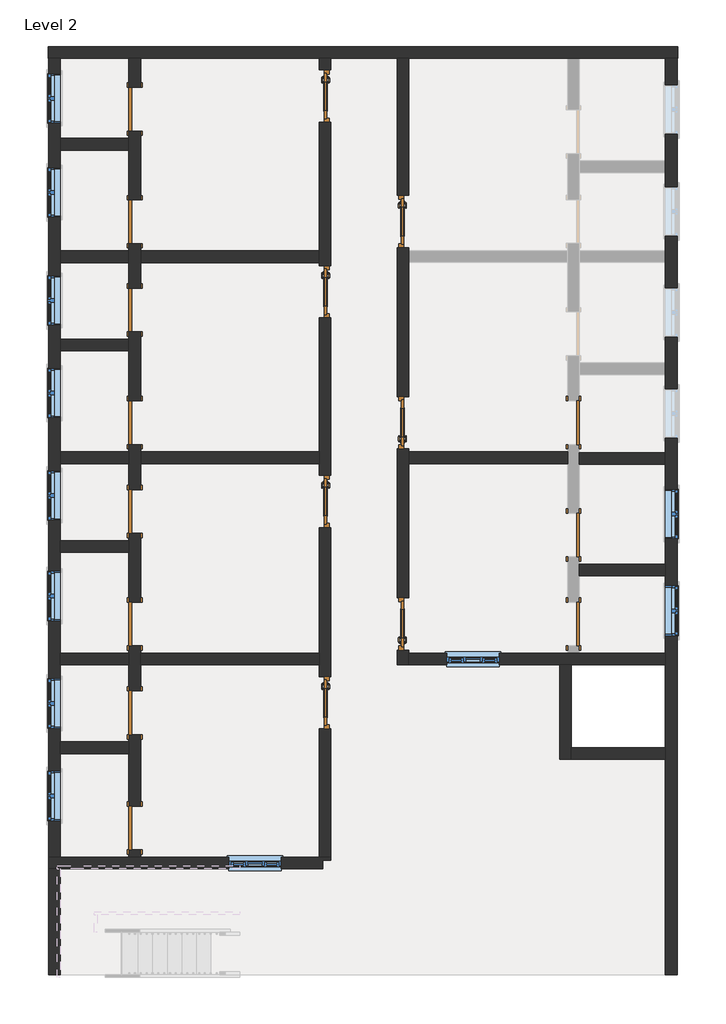
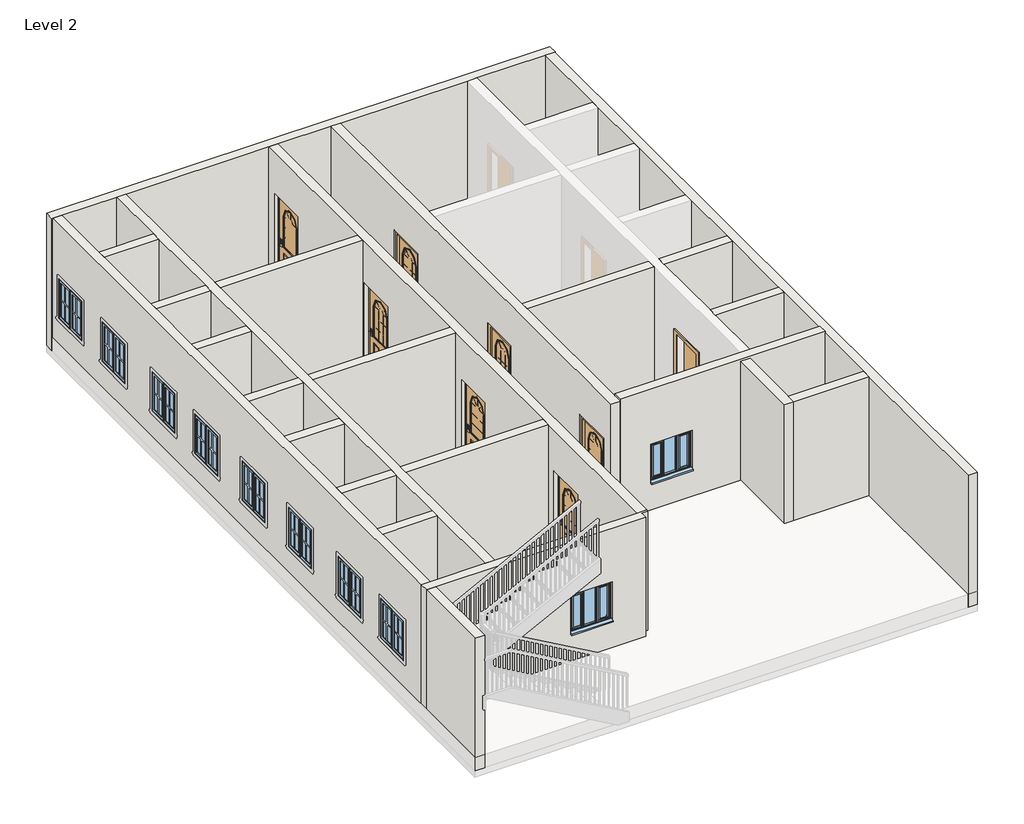
# One storey, part 1 of 4: 24 walls, 18 doors, 12 windows.
"""IFC4 building model written with IfcOpenShell, lengths in millimetres."""

from ifc_helpers import new_model, si_unit, frame, origin, place, context, project, spatial, polyline, outline, extrude, faceted_brep, transform, mapped, element, save
from components import doors_extsgl_w_glazing_bars_arched_910x2110mm_1ab485ba, doors_extsgl_w_glazing_bars_arched_910x2110mm_97dcda8a, door_fadea3f2, door_53b1b562, window_c29befe5, windows_tpl_plain_910x910mm_84e79c20

model = new_model("IFC4")

# Units and contexts
model_context = context("Model", 3, world=origin())
ifc_project = project(units=[si_unit("LENGTHUNIT", "METRE", prefix="MILLI")], contexts=[model_context])

# Site, building, storey
site = spatial("IfcSite", under=ifc_project)
building = spatial("IfcBuilding", under=site)
storey = spatial("IfcBuildingStorey", under=building, Name="Level 2", Elevation=3048.0)

# Doors
placement = place(None, origin())
doors_extsgl_w_glazing_bars_arched_910x2110mm_shape = doors_extsgl_w_glazing_bars_arched_910x2110mm_1ab485ba(model_context)
element("IfcDoor", 1, ObjectType="Doors_ExtSgl_w-Glazing_Bars_Arched : 910x2110mm", at=placement, inside=storey, context=model_context, shape_type="MappedRepresentation", body=[
    mapped(doors_extsgl_w_glazing_bars_arched_910x2110mm_shape, transform((-1635.1108866, 7135.2399728, 3048.0), x_axis=(0.0, -1.0, 0.0), y_axis=(1.0, 0.0, 0.0), z_axis=(0.0, 0.0, 1.0))),
])
element("IfcDoor", 2, ObjectType="Doors_ExtSgl_w-Glazing_Bars_Arched : 910x2110mm", at=placement, inside=storey, context=model_context, shape_type="MappedRepresentation", body=[
    mapped(doors_extsgl_w_glazing_bars_arched_910x2110mm_shape, transform((-1635.1108866, 3727.1935874, 3048.0), x_axis=(0.0, -1.0, 0.0), y_axis=(1.0, 0.0, 0.0), z_axis=(0.0, 0.0, 1.0))),
])
element("IfcDoor", 3, ObjectType="Doors_ExtSgl_w-Glazing_Bars_Arched : 910x2110mm", at=placement, inside=storey, context=model_context, shape_type="MappedRepresentation", body=[
    mapped(doors_extsgl_w_glazing_bars_arched_910x2110mm_shape, transform((-1635.1108866, 74.0399728, 3048.0), x_axis=(0.0, -1.0, 0.0), y_axis=(1.0, 0.0, 0.0), z_axis=(0.0, 0.0, 1.0))),
])
element("IfcDoor", 4, ObjectType="Doors_ExtSgl_w-Glazing_Bars_Arched : 910x2110mm", at=placement, inside=storey, context=model_context, shape_type="MappedRepresentation", body=[
    mapped(doors_extsgl_w_glazing_bars_arched_910x2110mm_shape, transform((-1635.1108866, -3431.1600272, 3048.0), x_axis=(0.0, -1.0, 0.0), y_axis=(1.0, 0.0, 0.0), z_axis=(0.0, 0.0, 1.0))),
])
element("IfcDoor", 5, ObjectType="Doors_ExtSgl_w-Glazing_Bars_Arched : 910x2110mm", at=placement, inside=storey, context=model_context, shape_type="MappedRepresentation", body=[
    mapped(doors_extsgl_w_glazing_bars_arched_910x2110mm_shape, transform((-276.2108866, -2059.5600272, 3048.0), x_axis=(0.0, 1.0, 0.0), y_axis=(-1.0, 0.0, 0.0), z_axis=(0.0, 0.0, 1.0))),
])
element("IfcDoor", 6, ObjectType="Doors_ExtSgl_w-Glazing_Bars_Arched : 910x2110mm", at=placement, inside=storey, context=model_context, shape_type="MappedRepresentation", body=[
    mapped(doors_extsgl_w_glazing_bars_arched_910x2110mm_shape, transform((-276.2108866, 1445.6399728, 3048.0), x_axis=(0.0, 1.0, 0.0), y_axis=(-1.0, 0.0, 0.0), z_axis=(0.0, 0.0, 1.0))),
])
doors_extsgl_w_glazing_bars_arched_910x2110mm_2_shape = doors_extsgl_w_glazing_bars_arched_910x2110mm_97dcda8a(model_context)
element("IfcDoor", 7, ObjectType="Doors_ExtSgl_w-Glazing_Bars_Arched : 910x2110mm", at=placement, inside=storey, context=model_context, shape_type="MappedRepresentation", body=[
    mapped(doors_extsgl_w_glazing_bars_arched_910x2110mm_2_shape, transform((-276.2108866, 4950.8399728, 3048.0), x_axis=(0.0, -1.0, 0.0), y_axis=(1.0, 0.0, 0.0), z_axis=(0.0, 0.0, 1.0))),
])
door_shape = door_fadea3f2(model_context)
element("IfcDoor", 8, ObjectType="Single-Flush : 30\" x 80\"", at=placement, inside=storey, context=model_context, shape_type="MappedRepresentation", body=[
    mapped(door_shape, transform((2695.5891134, -510.1600272, 3048.0), x_axis=(0.0, -1.0, 0.0), y_axis=(1.0, 0.0, 0.0), z_axis=(0.0, 0.0, 1.0))),
])
element("IfcDoor", 9, ObjectType="Single-Flush : 30\" x 80\"", at=placement, inside=storey, context=model_context, shape_type="MappedRepresentation", body=[
    mapped(door_shape, transform((2695.5891134, -2059.5600272, 3048.0), x_axis=(0.0, -1.0, 0.0), y_axis=(1.0, 0.0, 0.0), z_axis=(0.0, 0.0, 1.0))),
])
door_2_shape = door_53b1b562(model_context)
element("IfcDoor", 10, ObjectType="Single-Flush : 30\" x 80\"", at=placement, inside=storey, context=model_context, shape_type="MappedRepresentation", body=[
    mapped(door_2_shape, transform((-4949.8108866, 6906.6399728, 3048.0), x_axis=(0.0, -1.0, 0.0), y_axis=(1.0, 0.0, 0.0), z_axis=(0.0, 0.0, 1.0))),
])
element("IfcDoor", 11, ObjectType="Single-Flush : 30\" x 80\"", at=placement, inside=storey, context=model_context, shape_type="MappedRepresentation", body=[
    mapped(door_2_shape, transform((-4949.8108866, 4946.3935874, 3048.0), x_axis=(0.0, -1.0, 0.0), y_axis=(1.0, 0.0, 0.0), z_axis=(0.0, 0.0, 1.0))),
])
element("IfcDoor", 12, ObjectType="Single-Flush : 30\" x 80\"", at=placement, inside=storey, context=model_context, shape_type="MappedRepresentation", body=[
    mapped(door_2_shape, transform((-4949.8108866, 3407.538843, 3048.0), x_axis=(0.0, -1.0, 0.0), y_axis=(1.0, 0.0, 0.0), z_axis=(0.0, 0.0, 1.0))),
])
element("IfcDoor", 13, ObjectType="Single-Flush : 30\" x 80\"", at=placement, inside=storey, context=model_context, shape_type="MappedRepresentation", body=[
    mapped(door_2_shape, transform((-4949.8108866, 1445.6399728, 3048.0), x_axis=(0.0, -1.0, 0.0), y_axis=(1.0, 0.0, 0.0), z_axis=(0.0, 0.0, 1.0))),
])
element("IfcDoor", 14, ObjectType="Single-Flush : 30\" x 80\"", at=placement, inside=storey, context=model_context, shape_type="MappedRepresentation", body=[
    mapped(door_2_shape, transform((-4949.8108866, -103.7600272, 3048.0), x_axis=(0.0, -1.0, 0.0), y_axis=(1.0, 0.0, 0.0), z_axis=(0.0, 0.0, 1.0))),
])
element("IfcDoor", 15, ObjectType="Single-Flush : 30\" x 80\"", at=placement, inside=storey, context=model_context, shape_type="MappedRepresentation", body=[
    mapped(door_2_shape, transform((-4949.8108866, -2059.5600272, 3048.0), x_axis=(0.0, -1.0, 0.0), y_axis=(1.0, 0.0, 0.0), z_axis=(0.0, 0.0, 1.0))),
])
element("IfcDoor", 16, ObjectType="Single-Flush : 30\" x 80\"", at=placement, inside=storey, context=model_context, shape_type="MappedRepresentation", body=[
    mapped(door_2_shape, transform((-4949.8108866, -3608.9600272, 3048.0), x_axis=(0.0, -1.0, 0.0), y_axis=(1.0, 0.0, 0.0), z_axis=(0.0, 0.0, 1.0))),
])
element("IfcDoor", 17, ObjectType="Single-Flush : 30\" x 80\"", at=placement, inside=storey, context=model_context, shape_type="MappedRepresentation", body=[
    mapped(door_2_shape, transform((-4949.8108866, -5615.5600272, 3048.0), x_axis=(0.0, -1.0, 0.0), y_axis=(1.0, 0.0, 0.0), z_axis=(0.0, 0.0, 1.0))),
])
element("IfcDoor", 18, ObjectType="Single-Flush : 30\" x 80\"", at=placement, inside=storey, context=model_context, shape_type="MappedRepresentation", body=[
    mapped(door_2_shape, transform((2695.5891134, 1445.6399728, 3048.0), x_axis=(0.0, 1.0, 0.0), y_axis=(-1.0, 0.0, 0.0), z_axis=(0.0, 0.0, 1.0))),
])

# Walls
element("IfcWall", 19, ObjectType="4.5\" p", at=placement, inside=storey, context=model_context, shape_type="Brep", body=[
    faceted_brep([(-5051.4108866, -5996.5600272, 5080.0), (-5051.4108866, -5996.5600272, 3048.0), (-5051.4108866, -6123.5600272, 3048.0), (-5051.4108866, -6123.5600272, 6096.0), (-5051.4108866, -4320.1600272, 6096.0), (-5051.4108866, -4116.9600272, 6096.0), (-5051.4108866, -2770.7600272, 6096.0), (-5051.4108866, -2567.5600272, 6096.0), (-5051.4108866, -814.9600272, 6096.0), (-5051.4108866, -611.7600272, 6096.0), (-5051.4108866, 734.4399728, 6096.0), (-5051.4108866, 937.6399728, 6096.0), (-5051.4108866, 2696.338843, 6096.0), (-5051.4108866, 2899.538843, 6096.0), (-5051.4108866, 4235.1935874, 6096.0), (-5051.4108866, 4438.3935874, 6096.0), (-5051.4108866, 6195.4399728, 6096.0), (-5051.4108866, 6398.6399728, 6096.0), (-5051.4108866, 7795.6399728, 6096.0), (-5051.4108866, 7795.6399728, 3048.0), (-5051.4108866, 7287.6399728, 3048.0), (-5051.4108866, 7287.6399728, 5080.0), (-5051.4108866, 6525.6399728, 5080.0), (-5051.4108866, 6525.6399728, 3048.0), (-5051.4108866, 6398.6399728, 3048.0), (-5051.4108866, 6195.4399728, 3048.0), (-5051.4108866, 5327.3935874, 3048.0), (-5051.4108866, 5327.3935874, 5080.0), (-5051.4108866, 4565.3935874, 5080.0), (-5051.4108866, 4565.3935874, 3048.0), (-5051.4108866, 4438.3935874, 3048.0), (-5051.4108866, 4235.1935874, 3048.0), (-5051.4108866, 3788.538843, 3048.0), (-5051.4108866, 3788.538843, 5080.0), (-5051.4108866, 3026.538843, 5080.0), (-5051.4108866, 3026.538843, 3048.0), (-5051.4108866, 2899.538843, 3048.0), (-5051.4108866, 2696.338843, 3048.0), (-5051.4108866, 1826.6399728, 3048.0), (-5051.4108866, 1826.6399728, 5080.0), (-5051.4108866, 1064.6399728, 5080.0), (-5051.4108866, 1064.6399728, 3048.0), (-5051.4108866, 937.6399728, 3048.0), (-5051.4108866, 734.4399728, 3048.0), (-5051.4108866, 277.2399728, 3048.0), (-5051.4108866, 277.2399728, 5080.0), (-5051.4108866, -484.7600272, 5080.0), (-5051.4108866, -484.7600272, 3048.0), (-5051.4108866, -611.7600272, 3048.0), (-5051.4108866, -814.9600272, 3048.0), (-5051.4108866, -1678.5600272, 3048.0), (-5051.4108866, -1678.5600272, 5080.0), (-5051.4108866, -2440.5600272, 5080.0), (-5051.4108866, -2440.5600272, 3048.0), (-5051.4108866, -2567.5600272, 3048.0), (-5051.4108866, -2770.7600272, 3048.0), (-5051.4108866, -3227.9600272, 3048.0), (-5051.4108866, -3227.9600272, 5080.0), (-5051.4108866, -3989.9600272, 5080.0), (-5051.4108866, -3989.9600272, 3048.0), (-5051.4108866, -4116.9600272, 3048.0), (-5051.4108866, -4320.1600272, 3048.0), (-5051.4108866, -5234.5600272, 3048.0), (-5051.4108866, -5234.5600272, 5080.0), (-4848.2108866, -6123.5600272, 3048.0), (-4848.2108866, -5996.5600272, 3048.0), (-4848.2108866, -5996.5600272, 5080.0), (-4848.2108866, -5234.5600272, 5080.0), (-4848.2108866, -5234.5600272, 3048.0), (-4848.2108866, -3989.9600272, 3048.0), (-4848.2108866, -3989.9600272, 5080.0), (-4848.2108866, -3227.9600272, 5080.0), (-4848.2108866, -3227.9600272, 3048.0), (-4848.2108866, -2770.7600272, 3048.0), (-4848.2108866, -2567.5600272, 3048.0), (-4848.2108866, -2440.5600272, 3048.0), (-4848.2108866, -2440.5600272, 5080.0), (-4848.2108866, -1678.5600272, 5080.0), (-4848.2108866, -1678.5600272, 3048.0), (-4848.2108866, -484.7600272, 3048.0), (-4848.2108866, -484.7600272, 5080.0), (-4848.2108866, 277.2399728, 5080.0), (-4848.2108866, 277.2399728, 3048.0), (-4848.2108866, 734.4399728, 3048.0), (-4848.2108866, 937.6399728, 3048.0), (-4848.2108866, 1064.6399728, 3048.0), (-4848.2108866, 1064.6399728, 5080.0), (-4848.2108866, 1826.6399728, 5080.0), (-4848.2108866, 1826.6399728, 3048.0), (-4848.2108866, 3026.538843, 3048.0), (-4848.2108866, 3026.538843, 5080.0), (-4848.2108866, 3788.538843, 5080.0), (-4848.2108866, 3788.538843, 3048.0), (-4848.2108866, 4235.1935874, 3048.0), (-4848.2108866, 4438.3935874, 3048.0), (-4848.2108866, 4565.3935874, 3048.0), (-4848.2108866, 4565.3935874, 5080.0), (-4848.2108866, 5327.3935874, 5080.0), (-4848.2108866, 5327.3935874, 3048.0), (-4848.2108866, 6525.6399728, 3048.0), (-4848.2108866, 6525.6399728, 5080.0), (-4848.2108866, 7287.6399728, 5080.0), (-4848.2108866, 7287.6399728, 3048.0), (-4848.2108866, 7795.6399728, 3048.0), (-4848.2108866, 7795.6399728, 6096.0), (-4848.2108866, 4438.3935874, 6096.0), (-4848.2108866, 4235.1935874, 6096.0), (-4848.2108866, 937.6399728, 6096.0), (-4848.2108866, 734.4399728, 6096.0), (-4848.2108866, -2567.5600272, 6096.0), (-4848.2108866, -2770.7600272, 6096.0), (-4848.2108866, -6123.5600272, 6096.0)], [[[0, 1, 2, 3, 4, 5, 6, 7, 8, 9, 10, 11, 12, 13, 14, 15, 16, 17, 18, 19, 20, 21, 22, 23, 24, 25, 26, 27, 28, 29, 30, 31, 32, 33, 34, 35, 36, 37, 38, 39, 40, 41, 42, 43, 44, 45, 46, 47, 48, 49, 50, 51, 52, 53, 54, 55, 56, 57, 58, 59, 60, 61, 62, 63]], [[64, 65, 66, 67, 68, 69, 70, 71, 72, 73, 74, 75, 76, 77, 78, 79, 80, 81, 82, 83, 84, 85, 86, 87, 88, 89, 90, 91, 92, 93, 94, 95, 96, 97, 98, 99, 100, 101, 102, 103, 104, 105, 106, 107, 108, 109, 110, 111]], [[20, 19, 103, 102]], [[26, 25, 24, 23, 99, 98]], [[32, 31, 30, 29, 95, 94, 93, 92]], [[38, 37, 36, 35, 89, 88]], [[44, 43, 42, 41, 85, 84, 83, 82]], [[50, 49, 48, 47, 79, 78]], [[56, 55, 54, 53, 75, 74, 73, 72]], [[2, 1, 65, 64]], [[62, 61, 60, 59, 69, 68]], [[18, 17, 16, 15, 14, 13, 12, 11, 10, 9, 8, 7, 6, 5, 4, 3, 111, 110, 109, 108, 107, 106, 105, 104]], [[19, 18, 104, 103]], [[3, 2, 64, 111]], [[100, 99, 23, 22]], [[101, 100, 22, 21]], [[102, 101, 21, 20]], [[96, 95, 29, 28]], [[97, 96, 28, 27]], [[98, 97, 27, 26]], [[90, 89, 35, 34]], [[91, 90, 34, 33]], [[92, 91, 33, 32]], [[86, 85, 41, 40]], [[87, 86, 40, 39]], [[88, 87, 39, 38]], [[80, 79, 47, 46]], [[81, 80, 46, 45]], [[82, 81, 45, 44]], [[76, 75, 53, 52]], [[77, 76, 52, 51]], [[78, 77, 51, 50]], [[70, 69, 59, 58]], [[71, 70, 58, 57]], [[72, 71, 57, 56]], [[66, 65, 1, 0]], [[67, 66, 0, 63]], [[68, 67, 63, 62]]]),
])
element("IfcWall", 20, ObjectType="4.5\" p", at=placement, inside=storey, context=model_context, shape_type="SweptSolid", body=[
    extrude(outline(polyline([(-5051.4108866, 6195.4399728), (-6245.2108866, 6195.4399728), (-6245.2108866, 6398.6399728), (-5051.4108866, 6398.6399728), (-5051.4108866, 6195.4399728)])), frame((0.0, 0.0, 3048.0), z_axis=(0.0, 0.0, 1.0), x_axis=(1.0, 0.0, 0.0)), (0.0, 0.0, 1.0), 3048.0),
])
element("IfcWall", 21, ObjectType="4.5\" p", at=placement, inside=storey, context=model_context, shape_type="SweptSolid", body=[
    extrude(outline(polyline([(-5051.4108866, 4235.1935874), (-6245.2108866, 4235.1935874), (-6245.2108866, 4438.3935874), (-5051.4108866, 4438.3935874), (-5051.4108866, 4235.1935874)])), frame((0.0, 0.0, 3048.0), z_axis=(0.0, 0.0, 1.0), x_axis=(1.0, 0.0, 0.0)), (0.0, 0.0, 1.0), 3048.0),
])
element("IfcWall", 22, ObjectType="4.5\" p", at=placement, inside=storey, context=model_context, shape_type="SweptSolid", body=[
    extrude(outline(polyline([(-5051.4108866, 2696.338843), (-6245.2108866, 2696.338843), (-6245.2108866, 2899.538843), (-5051.4108866, 2899.538843), (-5051.4108866, 2696.338843)])), frame((0.0, 0.0, 3048.0), z_axis=(0.0, 0.0, 1.0), x_axis=(1.0, 0.0, 0.0)), (0.0, 0.0, 1.0), 3048.0),
])
element("IfcWall", 23, ObjectType="4.5\" p", at=placement, inside=storey, context=model_context, shape_type="SweptSolid", body=[
    extrude(outline(polyline([(-5051.4108866, 734.4399728), (-6245.2108866, 734.4399728), (-6245.2108866, 937.6399728), (-5051.4108866, 937.6399728), (-5051.4108866, 734.4399728)])), frame((0.0, 0.0, 3048.0), z_axis=(0.0, 0.0, 1.0), x_axis=(1.0, 0.0, 0.0)), (0.0, 0.0, 1.0), 3048.0),
])
element("IfcWall", 24, ObjectType="4.5\" p", at=placement, inside=storey, context=model_context, shape_type="SweptSolid", body=[
    extrude(outline(polyline([(-5051.4108866, -814.9600272), (-6245.2108866, -814.9600272), (-6245.2108866, -611.7600272), (-5051.4108866, -611.7600272), (-5051.4108866, -814.9600272)])), frame((0.0, 0.0, 3048.0), z_axis=(0.0, 0.0, 1.0), x_axis=(1.0, 0.0, 0.0)), (0.0, 0.0, 1.0), 3048.0),
])
element("IfcWall", 25, ObjectType="4.5\" p", at=placement, inside=storey, context=model_context, shape_type="SweptSolid", body=[
    extrude(outline(polyline([(-5051.4108866, -2770.7600272), (-6245.2108866, -2770.7600272), (-6245.2108866, -2567.5600272), (-5051.4108866, -2567.5600272), (-5051.4108866, -2770.7600272)])), frame((0.0, 0.0, 3048.0), z_axis=(0.0, 0.0, 1.0), x_axis=(1.0, 0.0, 0.0)), (0.0, 0.0, 1.0), 3048.0),
])
element("IfcWall", 26, ObjectType="4.5\" p", at=placement, inside=storey, context=model_context, shape_type="SweptSolid", body=[
    extrude(outline(polyline([(-5051.4108866, -4320.1600272), (-6245.2108866, -4320.1600272), (-6245.2108866, -4116.9600272), (-5051.4108866, -4116.9600272), (-5051.4108866, -4320.1600272)])), frame((0.0, 0.0, 3048.0), z_axis=(0.0, 0.0, 1.0), x_axis=(1.0, 0.0, 0.0)), (0.0, 0.0, 1.0), 3048.0),
])
element("IfcWall", 27, ObjectType="4.5\" p", at=placement, inside=storey, context=model_context, shape_type="Brep", body=[
    faceted_brep([(-1736.7108866, -3886.1600272, 5158.0), (-1736.7108866, -3886.1600272, 3048.0), (-1736.7108866, -6123.5600272, 3048.0), (-1736.7108866, -6123.5600272, 6096.0), (-1736.7108866, -2770.7600272, 6096.0), (-1736.7108866, -2567.5600272, 6096.0), (-1736.7108866, 734.4399728, 6096.0), (-1736.7108866, 937.6399728, 6096.0), (-1736.7108866, 4235.1935874, 6096.0), (-1736.7108866, 4438.3935874, 6096.0), (-1736.7108866, 7795.6399728, 6096.0), (-1736.7108866, 7795.6399728, 3048.0), (-1736.7108866, 7590.2399728, 3048.0), (-1736.7108866, 7590.2399728, 5158.0), (-1736.7108866, 6680.2399728, 5158.0), (-1736.7108866, 6680.2399728, 3048.0), (-1736.7108866, 4438.3935874, 3048.0), (-1736.7108866, 4235.1935874, 3048.0), (-1736.7108866, 4182.1935874, 3048.0), (-1736.7108866, 4182.1935874, 5158.0), (-1736.7108866, 3272.1935874, 5158.0), (-1736.7108866, 3272.1935874, 3048.0), (-1736.7108866, 937.6399728, 3048.0), (-1736.7108866, 734.4399728, 3048.0), (-1736.7108866, 529.0399728, 3048.0), (-1736.7108866, 529.0399728, 5158.0), (-1736.7108866, -380.9600272, 5158.0), (-1736.7108866, -380.9600272, 3048.0), (-1736.7108866, -2567.5600272, 3048.0), (-1736.7108866, -2770.7600272, 3048.0), (-1736.7108866, -2976.1600272, 3048.0), (-1736.7108866, -2976.1600272, 5158.0), (-1533.5108866, -6123.5600272, 3048.0), (-1533.5108866, -3886.1600272, 3048.0), (-1533.5108866, -3886.1600272, 5158.0), (-1533.5108866, -2976.1600272, 5158.0), (-1533.5108866, -2976.1600272, 3048.0), (-1533.5108866, -380.9600272, 3048.0), (-1533.5108866, -380.9600272, 5158.0), (-1533.5108866, 529.0399728, 5158.0), (-1533.5108866, 529.0399728, 3048.0), (-1533.5108866, 3272.1935874, 3048.0), (-1533.5108866, 3272.1935874, 5158.0), (-1533.5108866, 4182.1935874, 5158.0), (-1533.5108866, 4182.1935874, 3048.0), (-1533.5108866, 6680.2399728, 3048.0), (-1533.5108866, 6680.2399728, 5158.0), (-1533.5108866, 7590.2399728, 5158.0), (-1533.5108866, 7590.2399728, 3048.0), (-1533.5108866, 7795.6399728, 3048.0), (-1533.5108866, 7795.6399728, 6096.0), (-1533.5108866, -6123.5600272, 6096.0)], [[[0, 1, 2, 3, 4, 5, 6, 7, 8, 9, 10, 11, 12, 13, 14, 15, 16, 17, 18, 19, 20, 21, 22, 23, 24, 25, 26, 27, 28, 29, 30, 31]], [[32, 33, 34, 35, 36, 37, 38, 39, 40, 41, 42, 43, 44, 45, 46, 47, 48, 49, 50, 51]], [[12, 11, 49, 48]], [[18, 17, 16, 15, 45, 44]], [[24, 23, 22, 21, 41, 40]], [[2, 1, 33, 32]], [[30, 29, 28, 27, 37, 36]], [[10, 9, 8, 7, 6, 5, 4, 3, 51, 50]], [[3, 2, 32, 51]], [[11, 10, 50, 49]], [[48, 47, 13, 12]], [[46, 45, 15, 14]], [[47, 46, 14, 13]], [[44, 43, 19, 18]], [[42, 41, 21, 20]], [[43, 42, 20, 19]], [[40, 39, 25, 24]], [[38, 37, 27, 26]], [[39, 38, 26, 25]], [[36, 35, 31, 30]], [[34, 33, 1, 0]], [[35, 34, 0, 31]]]),
])
element("IfcWall", 28, ObjectType="4.5\" p", at=placement, inside=storey, context=model_context, shape_type="SweptSolid", body=[
    extrude(outline(polyline([(-1736.7108866, 4235.1935874), (-4848.2108866, 4235.1935874), (-4848.2108866, 4438.3935874), (-1736.7108866, 4438.3935874), (-1736.7108866, 4235.1935874)])), frame((0.0, 0.0, 3048.0), z_axis=(0.0, 0.0, 1.0), x_axis=(1.0, 0.0, 0.0)), (0.0, 0.0, 1.0), 3048.0),
])
element("IfcWall", 29, ObjectType="4.5\" p", at=placement, inside=storey, context=model_context, shape_type="SweptSolid", body=[
    extrude(outline(polyline([(-1736.7108866, 734.4399728), (-4848.2108866, 734.4399728), (-4848.2108866, 937.6399728), (-1736.7108866, 937.6399728), (-1736.7108866, 734.4399728)])), frame((0.0, 0.0, 3048.0), z_axis=(0.0, 0.0, 1.0), x_axis=(1.0, 0.0, 0.0)), (0.0, 0.0, 1.0), 3048.0),
])
element("IfcWall", 30, ObjectType="4.5\" p", at=placement, inside=storey, context=model_context, shape_type="SweptSolid", body=[
    extrude(outline(polyline([(-1736.7108866, -2770.7600272), (-4848.2108866, -2770.7600272), (-4848.2108866, -2567.5600272), (-1736.7108866, -2567.5600272), (-1736.7108866, -2770.7600272)])), frame((0.0, 0.0, 3048.0), z_axis=(0.0, 0.0, 1.0), x_axis=(1.0, 0.0, 0.0)), (0.0, 0.0, 1.0), 3048.0),
])
element("IfcWall", 31, ObjectType="4.5\" p", at=placement, inside=storey, context=model_context, shape_type="Brep", body=[
    faceted_brep([(-377.8108866, 4495.8399728, 5158.0), (-377.8108866, 4495.8399728, 3048.0), (-377.8108866, 1900.6399728, 3048.0), (-377.8108866, 1900.6399728, 5158.0), (-377.8108866, 990.6399728, 5158.0), (-377.8108866, 990.6399728, 3048.0), (-377.8108866, -1604.5600272, 3048.0), (-377.8108866, -1604.5600272, 5158.0), (-377.8108866, -2514.5600272, 5158.0), (-377.8108866, -2514.5600272, 3048.0), (-377.8108866, -2770.7600272, 3048.0), (-377.8108866, -2770.7600272, 6096.0), (-377.8108866, 7795.6399728, 6096.0), (-377.8108866, 7795.6399728, 3048.0), (-377.8108866, 5405.8399728, 3048.0), (-377.8108866, 5405.8399728, 5158.0), (-174.6108866, 1900.6399728, 3048.0), (-174.6108866, 4239.6399728, 3048.0), (-174.6108866, 4442.8399728, 3048.0), (-174.6108866, 4495.8399728, 3048.0), (-174.6108866, 4495.8399728, 5158.0), (-174.6108866, 5405.8399728, 5158.0), (-174.6108866, 5405.8399728, 3048.0), (-174.6108866, 7795.6399728, 3048.0), (-174.6108866, 7795.6399728, 6096.0), (-174.6108866, 4442.8399728, 6096.0), (-174.6108866, 4239.6399728, 6096.0), (-174.6108866, 937.6399728, 6096.0), (-174.6108866, 734.4399728, 6096.0), (-174.6108866, -2770.7600272, 6096.0), (-174.6108866, -2770.7600272, 3048.0), (-174.6108866, -2567.5600272, 3048.0), (-174.6108866, -2514.5600272, 3048.0), (-174.6108866, -2514.5600272, 5158.0), (-174.6108866, -1604.5600272, 5158.0), (-174.6108866, -1604.5600272, 3048.0), (-174.6108866, 734.4399728, 3048.0), (-174.6108866, 937.6399728, 3048.0), (-174.6108866, 990.6399728, 3048.0), (-174.6108866, 990.6399728, 5158.0), (-174.6108866, 1900.6399728, 5158.0)], [[[0, 1, 2, 3, 4, 5, 6, 7, 8, 9, 10, 11, 12, 13, 14, 15]], [[16, 17, 18, 19, 20, 21, 22, 23, 24, 25, 26, 27, 28, 29, 30, 31, 32, 33, 34, 35, 36, 37, 38, 39, 40]], [[32, 31, 30, 10, 9]], [[38, 37, 36, 35, 6, 5]], [[14, 13, 23, 22]], [[2, 1, 19, 18, 17, 16]], [[12, 11, 29, 28, 27, 26, 25, 24]], [[13, 12, 24, 23]], [[11, 10, 30, 29]], [[9, 8, 33, 32]], [[7, 6, 35, 34]], [[8, 7, 34, 33]], [[5, 4, 39, 38]], [[3, 2, 16, 40]], [[4, 3, 40, 39]], [[22, 21, 15, 14]], [[20, 19, 1, 0]], [[21, 20, 0, 15]]]),
])
element("IfcWall", 32, ObjectType="4.5\" p", at=placement, inside=storey, context=model_context, shape_type="Brep", body=[
    faceted_brep([(-174.6108866, -2770.7600272, 3048.0), (2454.2891134, -2770.7600272, 3048.0), (2657.4891134, -2770.7600272, 3048.0), (4295.7891134, -2770.7600272, 3048.0), (4295.7891134, -2770.7600272, 6136.1226014), (-174.6108866, -2770.7600272, 6136.1226014), (-174.6108866, -2770.7600272, 6096.0), (1397.9891134, -2770.7600272, 4872.4), (1397.9891134, -2770.7600272, 3962.4), (487.9891134, -2770.7600272, 3962.4), (487.9891134, -2770.7600272, 4872.4), (-174.6108866, -2567.5600272, 3048.0), (-174.6108866, -2567.5600272, 6136.1226014), (4295.7891134, -2567.5600272, 6136.1226014), (4295.7891134, -2567.5600272, 3048.0), (2797.1891134, -2567.5600272, 3048.0), (2593.9891134, -2567.5600272, 3048.0), (1397.9891134, -2567.5600272, 4872.4), (487.9891134, -2567.5600272, 4872.4), (487.9891134, -2567.5600272, 3962.4), (1397.9891134, -2567.5600272, 3962.4)], [[[0, 1, 2, 3, 4, 5, 6], [7, 8, 9, 10]], [[11, 12, 13, 14, 15, 16], [17, 18, 19, 20]], [[3, 2, 1, 0, 11, 16, 15, 14]], [[5, 4, 13, 12]], [[0, 6, 5, 12, 11]], [[4, 3, 14, 13]], [[8, 7, 17, 20]], [[9, 8, 20, 19]], [[10, 9, 19, 18]], [[7, 10, 18, 17]]]),
])
element("IfcWall", 33, ObjectType="4.5\" p", at=placement, inside=storey, context=model_context, shape_type="Brep", body=[
    faceted_brep([(2454.2891134, -2770.7600272, 3048.0), (2454.2891134, -4421.7600272, 3048.0), (2454.2891134, -4421.7600272, 6096.0), (2454.2891134, -2770.7600272, 6096.0), (2657.4891134, -2770.7600272, 3048.0), (2657.4891134, -2770.7600272, 6096.0), (2657.4891134, -4218.5600272, 6096.0), (2657.4891134, -4421.7600272, 6096.0), (2657.4891134, -4421.7600272, 3048.0), (2657.4891134, -4218.5600272, 3048.0)], [[[0, 1, 2, 3]], [[4, 5, 6, 7, 8, 9]], [[1, 0, 4, 9, 8]], [[3, 2, 7, 6, 5]], [[0, 3, 5, 4]], [[2, 1, 8, 7]]]),
])
element("IfcWall", 34, ObjectType="4.5\" p", at=placement, inside=storey, context=model_context, shape_type="SweptSolid", body=[
    extrude(outline(polyline([(2657.4891134, -4218.5600272), (4295.7891134, -4218.5600272), (4295.7891134, -4421.7600272), (2657.4891134, -4421.7600272), (2657.4891134, -4218.5600272)])), frame((0.0, 0.0, 3048.0), z_axis=(0.0, 0.0, 1.0), x_axis=(1.0, 0.0, 0.0)), (0.0, 0.0, 1.0), 3048.0),
])
element("IfcWall", 35, ObjectType="4.5\" p", at=placement, inside=storey, context=model_context, shape_type="SweptSolid", body=[
    extrude(outline(polyline([(4295.7891134, 721.7399728), (2797.1891134, 721.7399728), (2797.1891134, 924.9399728), (4295.7891134, 924.9399728), (4295.7891134, 721.7399728)])), frame((0.0, 0.0, 3048.0), z_axis=(0.0, 0.0, 1.0), x_axis=(1.0, 0.0, 0.0)), (0.0, 0.0, 1.0), 3048.0),
])
element("IfcWall", 36, ObjectType="4.5\" p", at=placement, inside=storey, context=model_context, shape_type="SweptSolid", body=[
    extrude(outline(polyline([(4295.7891134, -1221.3600272), (2797.1891134, -1221.3600272), (2797.1891134, -1018.1600272), (4295.7891134, -1018.1600272), (4295.7891134, -1221.3600272)])), frame((0.0, 0.0, 3048.0), z_axis=(0.0, 0.0, 1.0), x_axis=(1.0, 0.0, 0.0)), (0.0, 0.0, 1.0), 3048.0),
])
element("IfcWall", 37, ObjectType="4.5\" p", at=placement, inside=storey, context=model_context, shape_type="SweptSolid", body=[
    extrude(outline(polyline([(2593.9891134, 734.4399728), (-174.6108866, 734.4399728), (-174.6108866, 937.6399728), (2593.9891134, 937.6399728), (2593.9891134, 734.4399728)])), frame((0.0, 0.0, 3048.0), z_axis=(0.0, 0.0, 1.0), x_axis=(1.0, 0.0, 0.0)), (0.0, 0.0, 1.0), 3048.0),
])
element("IfcWall", 38, ObjectType="4.5\" p", at=placement, inside=storey, context=model_context, shape_type="SweptSolid", body=[
    extrude(outline(polyline([(-6448.4108866, -8168.2600272), (-6448.4108866, -6326.7600272), (-6245.2108866, -6326.7600272), (-6245.2108866, -8168.2600272), (-6448.4108866, -8168.2600272)])), frame((0.0, 0.0, 3048.0), z_axis=(0.0, 0.0, 1.0), x_axis=(1.0, 0.0, 0.0)), (0.0, 0.0, 1.0), 3048.0),
])
element("IfcWall", 39, ObjectType="9\" w", at=placement, inside=storey, context=model_context, shape_type="Brep", body=[
    faceted_brep([(-6461.1108866, 7795.6399728, 3048.0), (-6448.4108866, 7795.6399728, 3048.0), (-6245.2108866, 7795.6399728, 3048.0), (-5051.4108866, 7795.6399728, 3048.0), (-4848.2108866, 7795.6399728, 3048.0), (-1736.7108866, 7795.6399728, 3048.0), (-1533.5108866, 7795.6399728, 3048.0), (-377.8108866, 7795.6399728, 3048.0), (-174.6108866, 7795.6399728, 3048.0), (2593.9891134, 7795.6399728, 3048.0), (2797.1891134, 7795.6399728, 3048.0), (4295.7891134, 7795.6399728, 3048.0), (4498.9891134, 7795.6399728, 3048.0), (4511.6891134, 7795.6399728, 3048.0), (4511.6891134, 7795.6399728, 6096.0), (4498.9891134, 7795.6399728, 6096.0), (4295.7891134, 7795.6399728, 6096.0), (2797.1891134, 7795.6399728, 6096.0), (2593.9891134, 7795.6399728, 6096.0), (-174.6108866, 7795.6399728, 6096.0), (-377.8108866, 7795.6399728, 6096.0), (-1533.5108866, 7795.6399728, 6096.0), (-1736.7108866, 7795.6399728, 6096.0), (-4848.2108866, 7795.6399728, 6096.0), (-5051.4108866, 7795.6399728, 6096.0), (-6245.2108866, 7795.6399728, 6096.0), (-6448.4108866, 7795.6399728, 6096.0), (-6461.1108866, 7795.6399728, 6096.0), (-6461.1108866, 7998.8399728, 3048.0), (-6461.1108866, 7998.8399728, 6096.0), (4511.6891134, 7998.8399728, 6096.0), (4511.6891134, 7998.8399728, 3048.0)], [[[0, 1, 2, 3, 4, 5, 6, 7, 8, 9, 10, 11, 12, 13, 14, 15, 16, 17, 18, 19, 20, 21, 22, 23, 24, 25, 26, 27]], [[28, 29, 30, 31]], [[13, 12, 11, 10, 9, 8, 7, 6, 5, 4, 3, 2, 1, 0, 28, 31]], [[14, 13, 31, 30]], [[27, 26, 25, 24, 23, 22, 21, 20, 19, 18, 17, 16, 15, 14, 30, 29]], [[0, 27, 29, 28]]]),
])
element("IfcWall", 40, ObjectType="9\" w", at=placement, inside=storey, context=model_context, shape_type="Brep", body=[
    faceted_brep([(-6448.4108866, -6326.7600272, 6096.0), (-6448.4108866, -6326.7600272, 3048.0), (-6245.2108866, -6326.7600272, 3048.0), (-1673.2108866, -6326.7600272, 3048.0), (-1673.2108866, -6326.7600272, 6096.0), (-6245.2108866, -6326.7600272, 6096.0), (-2399.3108866, -6326.7600272, 4872.4), (-2399.3108866, -6326.7600272, 3962.4), (-3309.3108866, -6326.7600272, 3962.4), (-3309.3108866, -6326.7600272, 4872.4), (-1533.5108866, -6123.5600272, 3048.0), (-1736.7108866, -6123.5600272, 3048.0), (-4848.2108866, -6123.5600272, 3048.0), (-5051.4108866, -6123.5600272, 3048.0), (-6245.2108866, -6123.5600272, 3048.0), (-6448.4108866, -6123.5600272, 3048.0), (-6448.4108866, -6123.5600272, 6096.0), (-6245.2108866, -6123.5600272, 6096.0), (-5051.4108866, -6123.5600272, 6096.0), (-4848.2108866, -6123.5600272, 6096.0), (-1736.7108866, -6123.5600272, 6096.0), (-1533.5108866, -6123.5600272, 6096.0), (-2399.3108866, -6123.5600272, 3962.4), (-2399.3108866, -6123.5600272, 4872.4), (-3309.3108866, -6123.5600272, 4872.4), (-3309.3108866, -6123.5600272, 3962.4), (-1533.5108866, -6174.3600272, 3048.0), (-1673.2108866, -6174.3600272, 3048.0), (-1673.2108866, -6174.3600272, 6096.0), (-1533.5108866, -6174.3600272, 6096.0)], [[[0, 1, 2, 3, 4, 5], [6, 7, 8, 9]], [[10, 11, 12, 13, 14, 15, 16, 17, 18, 19, 20, 21], [22, 23, 24, 25]], [[15, 14, 13, 12, 11, 10, 26, 27, 3, 2, 1]], [[21, 20, 19, 18, 17, 16, 0, 5, 4, 28, 29]], [[1, 0, 16, 15]], [[10, 21, 29, 26]], [[7, 6, 23, 22]], [[8, 7, 22, 25]], [[9, 8, 25, 24]], [[6, 9, 24, 23]], [[28, 27, 26, 29]], [[27, 28, 4, 3]]]),
])
element("IfcWall", 41, ObjectType="9\" w", at=placement, inside=storey, context=model_context, shape_type="Brep", body=[
    faceted_brep([(-6448.4108866, 7795.6399728, 3048.0), (-6448.4108866, -6123.5600272, 3048.0), (-6448.4108866, -6123.5600272, 6096.0), (-6448.4108866, 7795.6399728, 6096.0), (-6448.4108866, 7528.9399728, 4876.8), (-6448.4108866, 6665.3399728, 4876.8), (-6448.4108866, 6665.3399728, 3962.4), (-6448.4108866, 7528.9399728, 3962.4), (-6448.4108866, 5890.6399728, 4876.8), (-6448.4108866, 5027.0399728, 4876.8), (-6448.4108866, 5027.0399728, 3962.4), (-6448.4108866, 5890.6399728, 3962.4), (-6448.4108866, 4006.5935874, 4876.8), (-6448.4108866, 3142.9935874, 4876.8), (-6448.4108866, 3142.9935874, 3962.4), (-6448.4108866, 4006.5935874, 3962.4), (-6448.4108866, 2391.538843, 4876.8), (-6448.4108866, 1527.938843, 4876.8), (-6448.4108866, 1527.938843, 3962.4), (-6448.4108866, 2391.538843, 3962.4), (-6448.4108866, 607.4399728, 4876.8), (-6448.4108866, -256.1600272, 4876.8), (-6448.4108866, -256.1600272, 3962.4), (-6448.4108866, 607.4399728, 3962.4), (-6448.4108866, -1145.1600272, 4876.8), (-6448.4108866, -2008.7600272, 4876.8), (-6448.4108866, -2008.7600272, 3962.4), (-6448.4108866, -1145.1600272, 3962.4), (-6448.4108866, -3012.0600272, 4876.8), (-6448.4108866, -3875.6600272, 4876.8), (-6448.4108866, -3875.6600272, 3962.4), (-6448.4108866, -3012.0600272, 3962.4), (-6448.4108866, -4624.9600272, 4876.8), (-6448.4108866, -5488.5600272, 4876.8), (-6448.4108866, -5488.5600272, 3962.4), (-6448.4108866, -4624.9600272, 3962.4), (-6245.2108866, 7795.6399728, 3048.0), (-6245.2108866, 7795.6399728, 6096.0), (-6245.2108866, 6398.6399728, 6096.0), (-6245.2108866, 6195.4399728, 6096.0), (-6245.2108866, 4438.3935874, 6096.0), (-6245.2108866, 4235.1935874, 6096.0), (-6245.2108866, 2899.538843, 6096.0), (-6245.2108866, 2696.338843, 6096.0), (-6245.2108866, 937.6399728, 6096.0), (-6245.2108866, 734.4399728, 6096.0), (-6245.2108866, -611.7600272, 6096.0), (-6245.2108866, -814.9600272, 6096.0), (-6245.2108866, -2567.5600272, 6096.0), (-6245.2108866, -2770.7600272, 6096.0), (-6245.2108866, -4116.9600272, 6096.0), (-6245.2108866, -4320.1600272, 6096.0), (-6245.2108866, -6123.5600272, 6096.0), (-6245.2108866, -6123.5600272, 3048.0), (-6245.2108866, -4320.1600272, 3048.0), (-6245.2108866, -4116.9600272, 3048.0), (-6245.2108866, -2770.7600272, 3048.0), (-6245.2108866, -2567.5600272, 3048.0), (-6245.2108866, -814.9600272, 3048.0), (-6245.2108866, -611.7600272, 3048.0), (-6245.2108866, 734.4399728, 3048.0), (-6245.2108866, 937.6399728, 3048.0), (-6245.2108866, 2696.338843, 3048.0), (-6245.2108866, 2899.538843, 3048.0), (-6245.2108866, 4235.1935874, 3048.0), (-6245.2108866, 4438.3935874, 3048.0), (-6245.2108866, 6195.4399728, 3048.0), (-6245.2108866, 6398.6399728, 3048.0), (-6245.2108866, 7528.9399728, 4876.8), (-6245.2108866, 7528.9399728, 3962.4), (-6245.2108866, 6665.3399728, 3962.4), (-6245.2108866, 6665.3399728, 4876.8), (-6245.2108866, 5890.6399728, 4876.8), (-6245.2108866, 5890.6399728, 3962.4), (-6245.2108866, 5027.0399728, 3962.4), (-6245.2108866, 5027.0399728, 4876.8), (-6245.2108866, 4006.5935874, 4876.8), (-6245.2108866, 4006.5935874, 3962.4), (-6245.2108866, 3142.9935874, 3962.4), (-6245.2108866, 3142.9935874, 4876.8), (-6245.2108866, 2391.538843, 4876.8), (-6245.2108866, 2391.538843, 3962.4), (-6245.2108866, 1527.938843, 3962.4), (-6245.2108866, 1527.938843, 4876.8), (-6245.2108866, 607.4399728, 4876.8), (-6245.2108866, 607.4399728, 3962.4), (-6245.2108866, -256.1600272, 3962.4), (-6245.2108866, -256.1600272, 4876.8), (-6245.2108866, -1145.1600272, 4876.8), (-6245.2108866, -1145.1600272, 3962.4), (-6245.2108866, -2008.7600272, 3962.4), (-6245.2108866, -2008.7600272, 4876.8), (-6245.2108866, -3012.0600272, 4876.8), (-6245.2108866, -3012.0600272, 3962.4), (-6245.2108866, -3875.6600272, 3962.4), (-6245.2108866, -3875.6600272, 4876.8), (-6245.2108866, -4624.9600272, 4876.8), (-6245.2108866, -4624.9600272, 3962.4), (-6245.2108866, -5488.5600272, 3962.4), (-6245.2108866, -5488.5600272, 4876.8)], [[[0, 1, 2, 3], [4, 5, 6, 7], [8, 9, 10, 11], [12, 13, 14, 15], [16, 17, 18, 19], [20, 21, 22, 23], [24, 25, 26, 27], [28, 29, 30, 31], [32, 33, 34, 35]], [[36, 37, 38, 39, 40, 41, 42, 43, 44, 45, 46, 47, 48, 49, 50, 51, 52, 53, 54, 55, 56, 57, 58, 59, 60, 61, 62, 63, 64, 65, 66, 67], [68, 69, 70, 71], [72, 73, 74, 75], [76, 77, 78, 79], [80, 81, 82, 83], [84, 85, 86, 87], [88, 89, 90, 91], [92, 93, 94, 95], [96, 97, 98, 99]], [[1, 0, 36, 67, 66, 65, 64, 63, 62, 61, 60, 59, 58, 57, 56, 55, 54, 53]], [[3, 2, 52, 51, 50, 49, 48, 47, 46, 45, 44, 43, 42, 41, 40, 39, 38, 37]], [[2, 1, 53, 52]], [[0, 3, 37, 36]], [[69, 68, 4, 7]], [[70, 69, 7, 6]], [[71, 70, 6, 5]], [[68, 71, 5, 4]], [[73, 72, 8, 11]], [[74, 73, 11, 10]], [[75, 74, 10, 9]], [[72, 75, 9, 8]], [[77, 76, 12, 15]], [[78, 77, 15, 14]], [[79, 78, 14, 13]], [[76, 79, 13, 12]], [[81, 80, 16, 19]], [[82, 81, 19, 18]], [[83, 82, 18, 17]], [[80, 83, 17, 16]], [[85, 84, 20, 23]], [[86, 85, 23, 22]], [[87, 86, 22, 21]], [[84, 87, 21, 20]], [[89, 88, 24, 27]], [[90, 89, 27, 26]], [[91, 90, 26, 25]], [[88, 91, 25, 24]], [[93, 92, 28, 31]], [[94, 93, 31, 30]], [[95, 94, 30, 29]], [[92, 95, 29, 28]], [[97, 96, 32, 35]], [[98, 97, 35, 34]], [[99, 98, 34, 33]], [[96, 99, 33, 32]]]),
])
element("IfcWall", 42, ObjectType="9\" w", at=placement, inside=storey, context=model_context, shape_type="Brep", body=[
    faceted_brep([(4295.7891134, 7795.6399728, 3048.0), (4295.7891134, 6004.9399728, 3048.0), (4295.7891134, 5801.7399728, 3048.0), (4295.7891134, 4442.8399728, 3048.0), (4295.7891134, 4239.6399728, 3048.0), (4295.7891134, 2487.0399728, 3048.0), (4295.7891134, 2283.8399728, 3048.0), (4295.7891134, 924.9399728, 3048.0), (4295.7891134, 721.7399728, 3048.0), (4295.7891134, -1018.1600272, 3048.0), (4295.7891134, -1221.3600272, 3048.0), (4295.7891134, -2567.5600272, 3048.0), (4295.7891134, -2770.7600272, 3048.0), (4295.7891134, -4218.5600272, 3048.0), (4295.7891134, -4421.7600272, 3048.0), (4295.7891134, -8168.2600272, 3048.0), (4295.7891134, -8168.2600272, 6096.0), (4295.7891134, -4421.7600272, 6096.0), (4295.7891134, -4218.5600272, 6096.0), (4295.7891134, -1221.3600272, 6096.0), (4295.7891134, -1018.1600272, 6096.0), (4295.7891134, 721.7399728, 6096.0), (4295.7891134, 924.9399728, 6096.0), (4295.7891134, 2283.8399728, 6096.0), (4295.7891134, 2487.0399728, 6096.0), (4295.7891134, 4239.6399728, 6096.0), (4295.7891134, 4442.8399728, 6096.0), (4295.7891134, 5801.7399728, 6096.0), (4295.7891134, 6004.9399728, 6096.0), (4295.7891134, 7795.6399728, 6096.0), (4295.7891134, -2262.7600272, 4876.8), (4295.7891134, -2262.7600272, 3962.4), (4295.7891134, -1399.1600272, 3962.4), (4295.7891134, -1399.1600272, 4876.8), (4295.7891134, -580.0100272, 4876.8), (4295.7891134, -580.0100272, 3962.4), (4295.7891134, 283.5899728, 3962.4), (4295.7891134, 283.5899728, 4876.8), (4295.7891134, 1172.5899728, 4876.8), (4295.7891134, 1172.5899728, 3962.4), (4295.7891134, 2036.1899728, 3962.4), (4295.7891134, 2036.1899728, 4876.8), (4295.7891134, 2931.5399728, 4876.8), (4295.7891134, 2931.5399728, 3962.4), (4295.7891134, 3795.1399728, 3962.4), (4295.7891134, 3795.1399728, 4876.8), (4295.7891134, 4690.4899728, 4876.8), (4295.7891134, 4690.4899728, 3962.4), (4295.7891134, 5554.0899728, 3962.4), (4295.7891134, 5554.0899728, 4876.8), (4295.7891134, 6468.4899728, 4876.8), (4295.7891134, 6468.4899728, 3962.4), (4295.7891134, 7332.0899728, 3962.4), (4295.7891134, 7332.0899728, 4876.8), (4498.9891134, 7795.6399728, 3048.0), (4498.9891134, 7795.6399728, 6096.0), (4498.9891134, -8168.2600272, 6096.0), (4498.9891134, -8168.2600272, 3048.0), (4498.9891134, -2262.7600272, 4876.8), (4498.9891134, -1399.1600272, 4876.8), (4498.9891134, -1399.1600272, 3962.4), (4498.9891134, -2262.7600272, 3962.4), (4498.9891134, -580.0100272, 4876.8), (4498.9891134, 283.5899728, 4876.8), (4498.9891134, 283.5899728, 3962.4), (4498.9891134, -580.0100272, 3962.4), (4498.9891134, 1172.5899728, 4876.8), (4498.9891134, 2036.1899728, 4876.8), (4498.9891134, 2036.1899728, 3962.4), (4498.9891134, 1172.5899728, 3962.4), (4498.9891134, 2931.5399728, 4876.8), (4498.9891134, 3795.1399728, 4876.8), (4498.9891134, 3795.1399728, 3962.4), (4498.9891134, 2931.5399728, 3962.4), (4498.9891134, 4690.4899728, 4876.8), (4498.9891134, 5554.0899728, 4876.8), (4498.9891134, 5554.0899728, 3962.4), (4498.9891134, 4690.4899728, 3962.4), (4498.9891134, 6468.4899728, 4876.8), (4498.9891134, 7332.0899728, 4876.8), (4498.9891134, 7332.0899728, 3962.4), (4498.9891134, 6468.4899728, 3962.4)], [[[0, 1, 2, 3, 4, 5, 6, 7, 8, 9, 10, 11, 12, 13, 14, 15, 16, 17, 18, 19, 20, 21, 22, 23, 24, 25, 26, 27, 28, 29], [30, 31, 32, 33], [34, 35, 36, 37], [38, 39, 40, 41], [42, 43, 44, 45], [46, 47, 48, 49], [50, 51, 52, 53]], [[54, 55, 56, 57], [58, 59, 60, 61], [62, 63, 64, 65], [66, 67, 68, 69], [70, 71, 72, 73], [74, 75, 76, 77], [78, 79, 80, 81]], [[15, 14, 13, 12, 11, 10, 9, 8, 7, 6, 5, 4, 3, 2, 1, 0, 54, 57]], [[16, 15, 57, 56]], [[29, 28, 27, 26, 25, 24, 23, 22, 21, 20, 19, 18, 17, 16, 56, 55]], [[0, 29, 55, 54]], [[31, 30, 58, 61]], [[32, 31, 61, 60]], [[33, 32, 60, 59]], [[30, 33, 59, 58]], [[35, 34, 62, 65]], [[36, 35, 65, 64]], [[37, 36, 64, 63]], [[34, 37, 63, 62]], [[39, 38, 66, 69]], [[40, 39, 69, 68]], [[41, 40, 68, 67]], [[38, 41, 67, 66]], [[43, 42, 70, 73]], [[44, 43, 73, 72]], [[45, 44, 72, 71]], [[42, 45, 71, 70]], [[47, 46, 74, 77]], [[48, 47, 77, 76]], [[49, 48, 76, 75]], [[46, 49, 75, 74]], [[51, 50, 78, 81]], [[52, 51, 81, 80]], [[53, 52, 80, 79]], [[50, 53, 79, 78]]]),
])

# Windows
window_shape = window_c29befe5(model_context)
element("IfcWindow", 43, ObjectType="Window-Casement-Double : 34\" x 36\"", at=placement, inside=storey, context=model_context, shape_type="MappedRepresentation", body=[
    mapped(window_shape, transform((-6346.8108866, 7097.1399728, 3048.0), x_axis=(0.0, 1.0, 0.0), y_axis=(-1.0, 0.0, 0.0), z_axis=(0.0, 0.0, 1.0))),
])
element("IfcWindow", 44, ObjectType="Window-Casement-Double : 34\" x 36\"", at=placement, inside=storey, context=model_context, shape_type="MappedRepresentation", body=[
    mapped(window_shape, transform((-6346.8108866, 5458.8399728, 3048.0), x_axis=(0.0, 1.0, 0.0), y_axis=(-1.0, 0.0, 0.0), z_axis=(0.0, 0.0, 1.0))),
])
element("IfcWindow", 45, ObjectType="Window-Casement-Double : 34\" x 36\"", at=placement, inside=storey, context=model_context, shape_type="MappedRepresentation", body=[
    mapped(window_shape, transform((-6346.8108866, 3574.7935874, 3048.0), x_axis=(0.0, 1.0, 0.0), y_axis=(-1.0, 0.0, 0.0), z_axis=(0.0, 0.0, 1.0))),
])
element("IfcWindow", 46, ObjectType="Window-Casement-Double : 34\" x 36\"", at=placement, inside=storey, context=model_context, shape_type="MappedRepresentation", body=[
    mapped(window_shape, transform((-6346.8108866, 1959.738843, 3048.0), x_axis=(0.0, 1.0, 0.0), y_axis=(-1.0, 0.0, 0.0), z_axis=(0.0, 0.0, 1.0))),
])
element("IfcWindow", 47, ObjectType="Window-Casement-Double : 34\" x 36\"", at=placement, inside=storey, context=model_context, shape_type="MappedRepresentation", body=[
    mapped(window_shape, transform((-6346.8108866, 175.6399728, 3048.0), x_axis=(0.0, 1.0, 0.0), y_axis=(-1.0, 0.0, 0.0), z_axis=(0.0, 0.0, 1.0))),
])
element("IfcWindow", 48, ObjectType="Window-Casement-Double : 34\" x 36\"", at=placement, inside=storey, context=model_context, shape_type="MappedRepresentation", body=[
    mapped(window_shape, transform((-6346.8108866, -1576.9600272, 3048.0), x_axis=(0.0, 1.0, 0.0), y_axis=(-1.0, 0.0, 0.0), z_axis=(0.0, 0.0, 1.0))),
])
element("IfcWindow", 49, ObjectType="Window-Casement-Double : 34\" x 36\"", at=placement, inside=storey, context=model_context, shape_type="MappedRepresentation", body=[
    mapped(window_shape, transform((-6346.8108866, -3443.8600272, 3048.0), x_axis=(0.0, 1.0, 0.0), y_axis=(-1.0, 0.0, 0.0), z_axis=(0.0, 0.0, 1.0))),
])
element("IfcWindow", 50, ObjectType="Window-Casement-Double : 34\" x 36\"", at=placement, inside=storey, context=model_context, shape_type="MappedRepresentation", body=[
    mapped(window_shape, transform((-6346.8108866, -5056.7600272, 3048.0), x_axis=(0.0, 1.0, 0.0), y_axis=(-1.0, 0.0, 0.0), z_axis=(0.0, 0.0, 1.0))),
])
element("IfcWindow", 51, ObjectType="Window-Casement-Double : 34\" x 36\"", at=placement, inside=storey, context=model_context, shape_type="MappedRepresentation", body=[
    mapped(window_shape, transform((4397.3891134, -1830.9600272, 3048.0), x_axis=(0.0, -1.0, 0.0), y_axis=(1.0, 0.0, 0.0), z_axis=(0.0, 0.0, 1.0))),
])
element("IfcWindow", 52, ObjectType="Window-Casement-Double : 34\" x 36\"", at=placement, inside=storey, context=model_context, shape_type="MappedRepresentation", body=[
    mapped(window_shape, transform((4397.3891134, -148.2100272, 3048.0), x_axis=(0.0, -1.0, 0.0), y_axis=(1.0, 0.0, 0.0), z_axis=(0.0, 0.0, 1.0))),
])
windows_tpl_plain_910x910mm_shape = windows_tpl_plain_910x910mm_84e79c20(model_context)
element("IfcWindow", 53, ObjectType="Windows_Tpl_Plain : 910x910mm", at=placement, inside=storey, context=model_context, shape_type="MappedRepresentation", body=[
    mapped(windows_tpl_plain_910x910mm_shape, transform((516.3224468, -2660.7034594, 2762.4), x_axis=(-1.0, 0.0, 0.0), y_axis=(0.0, -1.0, 0.0), z_axis=(0.0, 0.0, 1.0))),
])
element("IfcWindow", 54, ObjectType="Windows_Tpl_Plain : 910x910mm", at=placement, inside=storey, context=model_context, shape_type="MappedRepresentation", body=[
    mapped(windows_tpl_plain_910x910mm_shape, transform((-3280.9775532, -6216.7034594, 2762.4), x_axis=(-1.0, 0.0, 0.0), y_axis=(0.0, -1.0, 0.0), z_axis=(0.0, 0.0, 1.0))),
])

save(model, "model.ifc")

# Revit data of these elements
# Type "Doors_ExtSgl_w-Glazing_Bars_Arched : 910x2110mm"
#   Type Mark = "19"
#   Type Comments = "External Single"
#   Operation = "SingleSwingRight"
#   Construction Type Id = "SGL"
#   Keynote = "L20"
#   Analytic Construction = "Large single-glazed windows"
#   Wrap Layers (Int) from Ext = 0' - 6.98819"
#   Wrap Layers (Ext) from Ext = 0' - 4.03543"
#   Visual Light Transmittance = 0.9
#   Thickness = 0' - 1.73228"
#   Solar Heat Gain Coefficient = 0.86
#   Rough Width = 2' - 11.82677"
#   Rough Height = 6' - 11.07087"
#   O/A Frame Width = 0' - 2.51969"
#   Heat Transfer Coefficient (U) = 0.979472 BTU/(h·ft²·°F)
#   Handle Z Distance = 3' - 5.33858"
#   Glazing Thickness = 0' - 0.94488"
#   FrameWidth = 0' - 1.65354"
#   FrameOffset - External = 0' - 0.98425"
#   FrameDepth = 0' - 3.50394"
#   Door Panel Width = 2' - 7.77165"
#   Door Panel Thickness = 0' - 1.73228"
#   Door Panel Height = 6' - 6.74016"
#   DONT CHANGE - Half Glazed Width = 0' - 9.98031"
#   DONT CHANGE - Glazed Width = 1' - 7.96063"
#   Cill Thickness = 0' - 2.14567"
#   Cill Projection = 0' - 1.1811"
#   Handle X Distance = 0' - 2.95276"
#   Height = 6' - 11.07087"
#   Structural Tolerance = 0' - 0.25591"
#   Tolerance = 0' - 0.11811"
#   Undercut = 0' - 0.15748"
#   Width = 2' - 11.82677"
#   Cill Extension = 0' - 0.98425"
#   Cavity Closer Width = 0' - 1.9685"
#   Cavity Closer Offset from Ext = 0' - 4.03543"
#   Cavity Closer Depth = 0' - 3.34646"
#   Vis - Ironmongery = yes
#   Vis - Glazing Bars = yes
#   Vis - Cavity Closers = yes
#   Define Thermal Properties by = 1
#   Function = 1
#   Material Glass = Door - Glazing
#   Material Glazing Bar = Door - Panel
#   Material Door = Door - Panel
#   Material Frame = Door - Frame/Mullion
#   Material Ironmongery = Door - Handle
#   Wall Closure = (empty or 0)
# Type "Single-Flush : 30\" x 80\""
#   Type Mark = "5"
#   Construction Type Id = "MDOOR"
#   Assembly Code = "C1020"
#   Analytic Construction = "Metal"
#   Thickness = 0' - 2"
#   Heat Transfer Coefficient (U) = 0.651978 BTU/(h·ft²·°F)
#   Height = 6' - 8"
#   Trim Projection Ext = 0' - 1"
#   Trim Projection Int = 0' - 1"
#   Trim Width = 0' - 3"
#   Width = 2' - 6"
#   Define Thermal Properties by = 1
#   Define Thermal Properties by = 1
#   Door Material = Door - Panel
#   Frame Material = Door - Frame
#   Visual Light Transmittance = 0
#   Solar Heat Gain Coefficient = 0
#   Function = (empty or 0)
#   Wall Closure = (empty or 0)
# Type "4.5\" p"
#   Assembly Code = "B2010"
#   Layers, outside or top first: 0' - 8" no material (function 1)
# Type "9\" w"
#   Assembly Code = "B2010"
#   Layers, outside or top first: 0' - 8" no material (function 1)
# Type "Window-Casement-Double : 34\" x 36\""
#   Type Mark = "14"
#   Fire Rating = "0.5h"
#   Assembly Code = "B2020100"
#   Analytic Construction = "Double glazing - domestic"
#   Frame Extension [instance default] = 0' - 0 1/4"
#   Window Inset [instance default] = 0' - 0"
#   Wall Thickness [instance default] = 0' - 6"
#   Interior Wall Closure [instance default] = 0' - 2 1/4"
#   Half Width = 1' - 5"
#   Visual Light Transmittance = 0.81
#   Thermal Resistance (R) = 1.8146 (h·ft²·°F)/BTU
#   Solar Heat Gain Coefficient = 0.76
#   Rough Width = 2' - 10 1/2"
#   Rough Height = 3' - 0 1/2"
#   Height = 3' - 0"
#   Heat Transfer Coefficient (U) = 0.5511 BTU/(h·ft²·°F)
#   Exterior Wall Closure [instance default] = 0' - 1 1/4"
#   Extension Jamb [instance default] = 0' - 2 1/4"
#   Default Sill Height = 3' - 0"
#   Width = 2' - 10"
#   Define Thermal Properties by = 0
#   Muntin Visibility = yes
#   Interior Trim Visibility [instance default] = yes
#   Exterior Trim Visibility [instance default] = yes
#   Extension Jamb Visibility [instance default] = yes
#   Interior Trim Material = Wood - Stained
#   Muntin Pattern = Muntin Pattern_2x2 : Muntin Pattern_2x2
#   Interior Trim = Trim-Window-Interior-Flat : Picture Frame
#   Interior Frame Material = Wood - Stained
#   Glass Panel Material = Glass
#   Exterior Trim Material = Clad - White
#   Exterior Trim = Trim-Window-Exterior-Flat : with Sill
#   Exterior Frame Material = Clad - White
#   Wall Closure = (empty or 0)
# Type "Windows_Tpl_Plain : 910x910mm"
#   Type Mark = "18"
#   Operation = "TriplePanelVertical"
#   Construction Type Id = "GSP4R"
#   Manufacturer = "Revit"
#   Keynote = "L10"
#   Analytic Construction = "1/8 in Pilkington single glazing"
#   Wrap Layers (Ext) from Ext = 0' - 4.03543"
#   Wrap Layers (Int) from Ext = 0' - 6.98819"
#   Window Board Projection = 0' - 0.98425"
#   Window Board Extension = 0' - 0.98425"
#   Visual Light Transmittance = 0.9
#   Solar Heat Gain Coefficient = 0.78
#   Rough Width = 2' - 11.82677"
#   Rough Height = 2' - 11.82677"
#   Height = 2' - 11.82677"
#   Width = 2' - 11.82677"
#   Heat Transfer Coefficient (U) = 0.6496 BTU/(h·ft²·°F)
#   Glazing Thickness = 0' - 0.94488"
#   FrameOffset - External = 0' - 1.9685"
#   Frame Depth = 0' - 2.55906"
#   Default Head Height = 6' - 11.07087"
#   Cill Depth = 0' - 3.44488"
#   Cavity Closer Width = 0' - 1.9685"
#   Cavity Closer Offset from Ext = 0' - 4.03543"
#   Cavity Closer Depth = 0' - 3.34646"
#   Vis - Cavity Closers = yes
#   Define Thermal Properties by = 1
#   Material Trim = Window Frame
#   Material Glass = Glass
#   Material Frame = Window Frame
#   Wall Closure = (empty or 0)
# Elements 1, 2, 3, 4, 5, 6, 7 (IfcDoor, "Doors_ExtSgl_w-Glazing_Bars_Arched : 910x2110mm")
#   Phase Created = New Construction
#   Materials on its faces: "Door - Panel", "Door - Handle", "Door - Frame/Mullion", "Door - Glazing"
# Elements 8, 9, 10, 11, 12, 13, 14, 15, 16, 17, 18 (IfcDoor, "Single-Flush : 30\" x 80\"")
#   Phase Created = New Construction
#   Materials on its faces: "Door - Frame", "Door - Panel"
# Elements 19, 20, 21, 22, 23, 24, 25, 26, 28, 29, 30, 35, 36, 37, 38 (IfcWall, "4.5\" p")
#   Top Offset = 0' - 0"
#   Base Offset = 0' - 0"
#   wall height = 10' - 0"
#   Phase Created = New Construction
#   Base Constraint = Level 2
#   Top Constraint = Level 3
#   Materials on its faces: "Default Wall"
# Element 27 (IfcWall, "4.5\" p")
#   Top Offset = 0' - 0"
#   Base Offset = 0' - 0"
#   wall height = 10' - 0"
#   Phase Created = New Construction
#   Base Constraint = Level 2
#   Top Constraint = Level 3
#   Materials on its faces: "Default Wall", "Brick, Common"
# Element 31 (IfcWall, "4.5\" p")
#   Top Offset = 0' - 0"
#   Base Offset = 0' - 0"
#   wall height = 10' - 0"
#   Phase Created = New Construction
#   Base Constraint = Level 2
#   Top Constraint = Level 3
#   Materials on its faces: "Default Wall", "Brick, Common", "Window Frame"
# Element 32 (IfcWall, "4.5\" p")
#   Top Offset = 0' - 1.57963"
#   Base Offset = 0' - 0"
#   wall height = 10' - 1.57963"
#   Phase Created = New Construction
#   Base Constraint = Level 2
#   Top Constraint = Level 3
#   Materials on its faces: "Default Wall", "Window Frame"
# Elements 33, 34 (IfcWall, "4.5\" p")
#   Top Offset = 0' - 0"
#   Base Offset = 0' - 0"
#   wall height = 10' - 0"
#   Phase Created = New Construction
#   Base Constraint = Level 2
#   Top Constraint = Level 3
#   Materials on its faces: "Default Wall", "Doors - Glazing Bars"
# Element 39 (IfcWall, "9\" w")
#   Top Offset = 0' - 0"
#   Base Offset = 0' - 0"
#   wall height = 10' - 0"
#   Phase Created = New Construction
#   Base Constraint = Level 2
#   Top Constraint = Level 3
#   Materials on its faces: "Default Wall", "Cherry", "Wood - Stained"
# Element 40 (IfcWall, "9\" w")
#   Top Offset = 0' - 0"
#   Base Offset = 0' - 0"
#   wall height = 10' - 0"
#   Phase Created = New Construction
#   Base Constraint = Level 2
#   Top Constraint = Level 3
#   Materials on its faces: "Default Wall", "Door - Frame/Mullion", "Door - Architrave"
# Element 41 (IfcWall, "9\" w")
#   Top Offset = 0' - 0"
#   Base Offset = 0' - 0"
#   wall height = 10' - 0"
#   Phase Created = New Construction
#   Base Constraint = Level 2
#   Top Constraint = Level 3
#   Materials on its faces: "Default Wall"
# Element 42 (IfcWall, "9\" w")
#   Top Offset = 0' - 0"
#   Base Offset = 0' - 0"
#   wall height = 10' - 0"
#   Phase Created = New Construction
#   Base Constraint = Level 2
#   Top Constraint = Level 3
#   Materials on its faces: "Default Wall", "Wood - Stained", "Earth"
